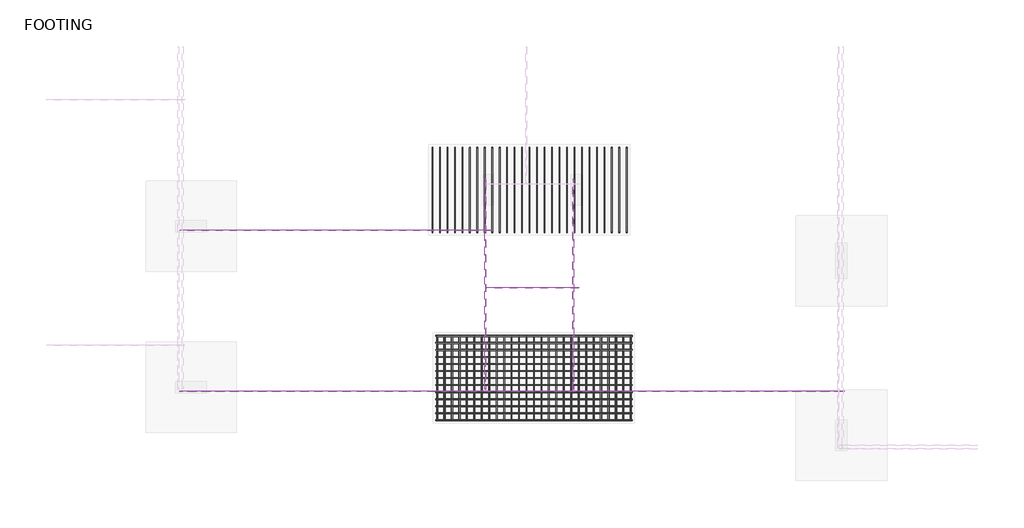
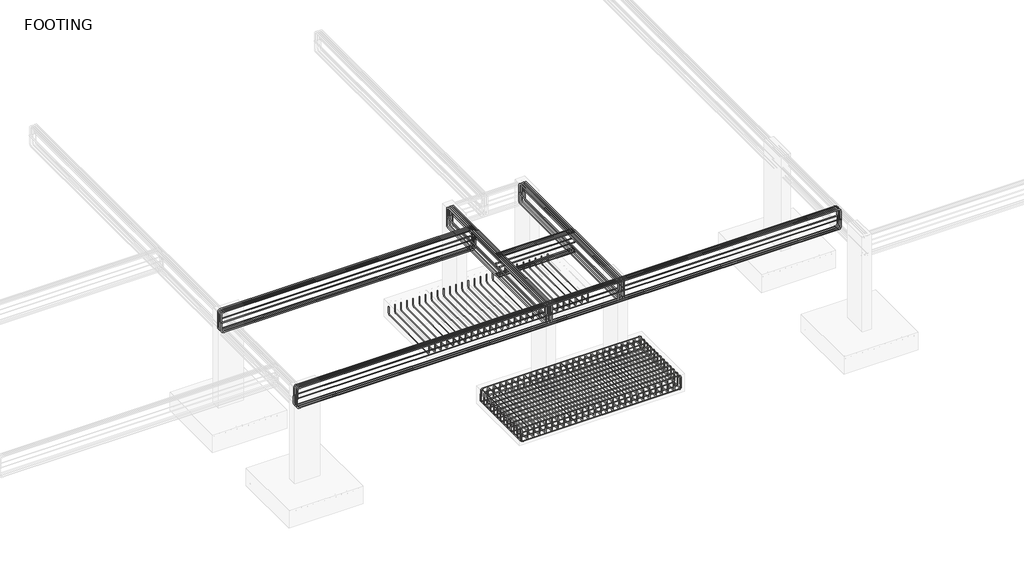
# One storey, part 3 of 12: 20 reinforcing bars.
"""IFC4 building model written with IfcOpenShell, lengths in millimetres."""

from ifc_helpers import new_model, si_unit, point, frame, origin, place, context, project, spatial, polyline, circle_curve, trimmed, segment, composite_curve, source, transform, mapped, element, save
from ifc_brep_helpers import swept_disk

model = new_model("IFC4")

# Units and contexts
model_context = context("Model", 3, world=origin())
ifc_project = project(units=[si_unit("LENGTHUNIT", "METRE", prefix="MILLI")], contexts=[model_context])

# Site, building, storey
site = spatial("IfcSite", under=ifc_project)
building = spatial("IfcBuilding", under=site)
storey = spatial("IfcBuildingStorey", under=building, Name="FOOTING", Elevation=-5638.8)

# Reinforcing bars
placement = place(None, origin())
reinforcing_bar_shape = source(origin(), model_context, "Body", "SolidModel", [
    swept_disk(composite_curve([segment(polyline([(-3549.5501665, -12181.7541655, -5831.4), (-3549.5501665, -12181.7541655, -5978.7)]), True, "CONTINUOUS"), segment(trimmed(circle_curve(frame((-3549.5501665, -12228.1041655, -5978.7), z_axis=(-1.0, 0.0, 0.0), x_axis=(0.0, 46.350000000000364, 0.0)), 46.35), [point((-3549.5501665, -12181.7541655, -5978.7))], [point((-3549.5501665, -12228.1041655, -6025.05))], True, "CARTESIAN"), True, "CONTINUOUS"), segment(polyline([(-3549.5501665, -12228.1041655, -6025.05), (-3549.5501665, -13822.7041655, -6025.05)]), True, "CONTINUOUS"), segment(trimmed(circle_curve(frame((-3549.5501665, -13822.7041655, -5978.7), z_axis=(-1.0, 0.0, 0.0), x_axis=(0.0, 0.0, -46.350000000000364)), 46.35), [point((-3549.5501665, -13822.7041655, -6025.05))], [point((-3549.5501665, -13869.0541655, -5978.7))], True, "CARTESIAN"), True, "CONTINUOUS"), segment(polyline([(-3549.5501665, -13869.0541655, -5978.7), (-3549.5501665, -13869.0541655, -5831.4)]), True, "CONTINUOUS")], self_intersect=False), 6.35),
])
element("IfcReinforcingBar", 1, at=placement, inside=storey, context=model_context, shape_type="MappedRepresentation", body=[
    mapped(reinforcing_bar_shape, transform((0.0, 0.0, 0.0), x_axis=(1.0, 0.0, 0.0), y_axis=(0.0, 1.0, 0.0), z_axis=(0.0, 0.0, 1.0))),
    mapped(reinforcing_bar_shape, transform((148.4113099, 0.0, 0.0), x_axis=(1.0, 0.0, 0.0), y_axis=(0.0, 1.0, 0.0), z_axis=(0.0, 0.0, 1.0))),
    mapped(reinforcing_bar_shape, transform((296.8226198, 0.0, 0.0), x_axis=(1.0, 0.0, 0.0), y_axis=(0.0, 1.0, 0.0), z_axis=(0.0, 0.0, 1.0))),
    mapped(reinforcing_bar_shape, transform((445.2339297, 0.0, 0.0), x_axis=(1.0, 0.0, 0.0), y_axis=(0.0, 1.0, 0.0), z_axis=(0.0, 0.0, 1.0))),
    mapped(reinforcing_bar_shape, transform((593.6452396, 0.0, 0.0), x_axis=(1.0, 0.0, 0.0), y_axis=(0.0, 1.0, 0.0), z_axis=(0.0, 0.0, 1.0))),
    mapped(reinforcing_bar_shape, transform((742.0565495, 0.0, 0.0), x_axis=(1.0, 0.0, 0.0), y_axis=(0.0, 1.0, 0.0), z_axis=(0.0, 0.0, 1.0))),
    mapped(reinforcing_bar_shape, transform((890.4678594, 0.0, 0.0), x_axis=(1.0, 0.0, 0.0), y_axis=(0.0, 1.0, 0.0), z_axis=(0.0, 0.0, 1.0))),
    mapped(reinforcing_bar_shape, transform((1038.8791693, 0.0, 0.0), x_axis=(1.0, 0.0, 0.0), y_axis=(0.0, 1.0, 0.0), z_axis=(0.0, 0.0, 1.0))),
    mapped(reinforcing_bar_shape, transform((1187.2904792, 0.0, 0.0), x_axis=(1.0, 0.0, 0.0), y_axis=(0.0, 1.0, 0.0), z_axis=(0.0, 0.0, 1.0))),
    mapped(reinforcing_bar_shape, transform((1335.7017891, 0.0, 0.0), x_axis=(1.0, 0.0, 0.0), y_axis=(0.0, 1.0, 0.0), z_axis=(0.0, 0.0, 1.0))),
    mapped(reinforcing_bar_shape, transform((1484.113099, 0.0, 0.0), x_axis=(1.0, 0.0, 0.0), y_axis=(0.0, 1.0, 0.0), z_axis=(0.0, 0.0, 1.0))),
    mapped(reinforcing_bar_shape, transform((1632.5244089, 0.0, 0.0), x_axis=(1.0, 0.0, 0.0), y_axis=(0.0, 1.0, 0.0), z_axis=(0.0, 0.0, 1.0))),
    mapped(reinforcing_bar_shape, transform((1780.9357188, 0.0, 0.0), x_axis=(1.0, 0.0, 0.0), y_axis=(0.0, 1.0, 0.0), z_axis=(0.0, 0.0, 1.0))),
    mapped(reinforcing_bar_shape, transform((1929.3470287, 0.0, 0.0), x_axis=(1.0, 0.0, 0.0), y_axis=(0.0, 1.0, 0.0), z_axis=(0.0, 0.0, 1.0))),
    mapped(reinforcing_bar_shape, transform((2077.7583386, 0.0, 0.0), x_axis=(1.0, 0.0, 0.0), y_axis=(0.0, 1.0, 0.0), z_axis=(0.0, 0.0, 1.0))),
    mapped(reinforcing_bar_shape, transform((2226.1696485, 0.0, 0.0), x_axis=(1.0, 0.0, 0.0), y_axis=(0.0, 1.0, 0.0), z_axis=(0.0, 0.0, 1.0))),
    mapped(reinforcing_bar_shape, transform((2374.5809584, 0.0, 0.0), x_axis=(1.0, 0.0, 0.0), y_axis=(0.0, 1.0, 0.0), z_axis=(0.0, 0.0, 1.0))),
    mapped(reinforcing_bar_shape, transform((2522.9922683, 0.0, 0.0), x_axis=(1.0, 0.0, 0.0), y_axis=(0.0, 1.0, 0.0), z_axis=(0.0, 0.0, 1.0))),
    mapped(reinforcing_bar_shape, transform((2671.4035782, 0.0, 0.0), x_axis=(1.0, 0.0, 0.0), y_axis=(0.0, 1.0, 0.0), z_axis=(0.0, 0.0, 1.0))),
    mapped(reinforcing_bar_shape, transform((2819.814888, 0.0, 0.0), x_axis=(1.0, 0.0, 0.0), y_axis=(0.0, 1.0, 0.0), z_axis=(0.0, 0.0, 1.0))),
    mapped(reinforcing_bar_shape, transform((2968.2261979, 0.0, 0.0), x_axis=(1.0, 0.0, 0.0), y_axis=(0.0, 1.0, 0.0), z_axis=(0.0, 0.0, 1.0))),
    mapped(reinforcing_bar_shape, transform((3116.6375078, 0.0, 0.0), x_axis=(1.0, 0.0, 0.0), y_axis=(0.0, 1.0, 0.0), z_axis=(0.0, 0.0, 1.0))),
    mapped(reinforcing_bar_shape, transform((3265.0488177, 0.0, 0.0), x_axis=(1.0, 0.0, 0.0), y_axis=(0.0, 1.0, 0.0), z_axis=(0.0, 0.0, 1.0))),
    mapped(reinforcing_bar_shape, transform((3413.4601276, 0.0, 0.0), x_axis=(1.0, 0.0, 0.0), y_axis=(0.0, 1.0, 0.0), z_axis=(0.0, 0.0, 1.0))),
    mapped(reinforcing_bar_shape, transform((3561.8714375, 0.0, 0.0), x_axis=(1.0, 0.0, 0.0), y_axis=(0.0, 1.0, 0.0), z_axis=(0.0, 0.0, 1.0))),
    mapped(reinforcing_bar_shape, transform((3710.2827474, 0.0, 0.0), x_axis=(1.0, 0.0, 0.0), y_axis=(0.0, 1.0, 0.0), z_axis=(0.0, 0.0, 1.0))),
    mapped(reinforcing_bar_shape, transform((3858.6940573, 0.0, 0.0), x_axis=(1.0, 0.0, 0.0), y_axis=(0.0, 1.0, 0.0), z_axis=(0.0, 0.0, 1.0))),
])
reinforcing_bar_2_shape = source(origin(), model_context, "Body", "SolidModel", [
    swept_disk(composite_curve([segment(polyline([(296.2067827, -12181.7541655, -5901.65), (296.2067827, -12181.7541655, -5754.35)]), True, "CONTINUOUS"), segment(trimmed(circle_curve(frame((296.2067827, -12228.1041655, -5754.35), z_axis=(1.0, 0.0, 0.0), x_axis=(0.0, 46.350000000000364, 0.0)), 46.35), [point((296.2067827, -12181.7541655, -5754.35))], [point((296.2067827, -12228.1041655, -5708.0))], True, "CARTESIAN"), True, "CONTINUOUS"), segment(polyline([(296.2067827, -12228.1041655, -5708.0), (296.2067827, -13822.7041655, -5708.0)]), True, "CONTINUOUS"), segment(trimmed(circle_curve(frame((296.2067827, -13822.7041655, -5754.35), z_axis=(1.0, 0.0, 0.0), x_axis=(0.0, 0.0, 46.350000000000364)), 46.35), [point((296.2067827, -13822.7041655, -5708.0))], [point((296.2067827, -13869.0541655, -5754.35))], True, "CARTESIAN"), True, "CONTINUOUS"), segment(polyline([(296.2067827, -13869.0541655, -5754.35), (296.2067827, -13869.0541655, -5901.65)]), True, "CONTINUOUS")], self_intersect=False), 6.35),
])
element("IfcReinforcingBar", 2, at=placement, inside=storey, context=model_context, shape_type="MappedRepresentation", body=[
    mapped(reinforcing_bar_2_shape, transform((0.0, 0.0, 0.0), x_axis=(1.0, 0.0, 0.0), y_axis=(0.0, 1.0, 0.0), z_axis=(0.0, 0.0, 1.0))),
    mapped(reinforcing_bar_2_shape, transform((-147.4810365, 0.0, 0.0), x_axis=(1.0, 0.0, 0.0), y_axis=(0.0, 1.0, 0.0), z_axis=(0.0, 0.0, 1.0))),
    mapped(reinforcing_bar_2_shape, transform((-294.962073, 0.0, 0.0), x_axis=(1.0, 0.0, 0.0), y_axis=(0.0, 1.0, 0.0), z_axis=(0.0, 0.0, 1.0))),
    mapped(reinforcing_bar_2_shape, transform((-442.4431095, 0.0, 0.0), x_axis=(1.0, 0.0, 0.0), y_axis=(0.0, 1.0, 0.0), z_axis=(0.0, 0.0, 1.0))),
    mapped(reinforcing_bar_2_shape, transform((-589.924146, 0.0, 0.0), x_axis=(1.0, 0.0, 0.0), y_axis=(0.0, 1.0, 0.0), z_axis=(0.0, 0.0, 1.0))),
    mapped(reinforcing_bar_2_shape, transform((-737.4051825, 0.0, 0.0), x_axis=(1.0, 0.0, 0.0), y_axis=(0.0, 1.0, 0.0), z_axis=(0.0, 0.0, 1.0))),
    mapped(reinforcing_bar_2_shape, transform((-884.886219, 0.0, 0.0), x_axis=(1.0, 0.0, 0.0), y_axis=(0.0, 1.0, 0.0), z_axis=(0.0, 0.0, 1.0))),
    mapped(reinforcing_bar_2_shape, transform((-1032.3672556, 0.0, 0.0), x_axis=(1.0, 0.0, 0.0), y_axis=(0.0, 1.0, 0.0), z_axis=(0.0, 0.0, 1.0))),
    mapped(reinforcing_bar_2_shape, transform((-1179.8482921, 0.0, 0.0), x_axis=(1.0, 0.0, 0.0), y_axis=(0.0, 1.0, 0.0), z_axis=(0.0, 0.0, 1.0))),
    mapped(reinforcing_bar_2_shape, transform((-1327.3293286, 0.0, 0.0), x_axis=(1.0, 0.0, 0.0), y_axis=(0.0, 1.0, 0.0), z_axis=(0.0, 0.0, 1.0))),
    mapped(reinforcing_bar_2_shape, transform((-1474.8103651, 0.0, 0.0), x_axis=(1.0, 0.0, 0.0), y_axis=(0.0, 1.0, 0.0), z_axis=(0.0, 0.0, 1.0))),
    mapped(reinforcing_bar_2_shape, transform((-1622.2914016, 0.0, 0.0), x_axis=(1.0, 0.0, 0.0), y_axis=(0.0, 1.0, 0.0), z_axis=(0.0, 0.0, 1.0))),
    mapped(reinforcing_bar_2_shape, transform((-1769.7724381, 0.0, 0.0), x_axis=(1.0, 0.0, 0.0), y_axis=(0.0, 1.0, 0.0), z_axis=(0.0, 0.0, 1.0))),
    mapped(reinforcing_bar_2_shape, transform((-1917.2534746, 0.0, 0.0), x_axis=(1.0, 0.0, 0.0), y_axis=(0.0, 1.0, 0.0), z_axis=(0.0, 0.0, 1.0))),
    mapped(reinforcing_bar_2_shape, transform((-2064.7345111, 0.0, 0.0), x_axis=(1.0, 0.0, 0.0), y_axis=(0.0, 1.0, 0.0), z_axis=(0.0, 0.0, 1.0))),
    mapped(reinforcing_bar_2_shape, transform((-2212.2155476, 0.0, 0.0), x_axis=(1.0, 0.0, 0.0), y_axis=(0.0, 1.0, 0.0), z_axis=(0.0, 0.0, 1.0))),
    mapped(reinforcing_bar_2_shape, transform((-2359.6965841, 0.0, 0.0), x_axis=(1.0, 0.0, 0.0), y_axis=(0.0, 1.0, 0.0), z_axis=(0.0, 0.0, 1.0))),
    mapped(reinforcing_bar_2_shape, transform((-2507.1776206, 0.0, 0.0), x_axis=(1.0, 0.0, 0.0), y_axis=(0.0, 1.0, 0.0), z_axis=(0.0, 0.0, 1.0))),
    mapped(reinforcing_bar_2_shape, transform((-2654.6586571, 0.0, 0.0), x_axis=(1.0, 0.0, 0.0), y_axis=(0.0, 1.0, 0.0), z_axis=(0.0, 0.0, 1.0))),
    mapped(reinforcing_bar_2_shape, transform((-2802.1396936, 0.0, 0.0), x_axis=(1.0, 0.0, 0.0), y_axis=(0.0, 1.0, 0.0), z_axis=(0.0, 0.0, 1.0))),
    mapped(reinforcing_bar_2_shape, transform((-2949.6207301, 0.0, 0.0), x_axis=(1.0, 0.0, 0.0), y_axis=(0.0, 1.0, 0.0), z_axis=(0.0, 0.0, 1.0))),
    mapped(reinforcing_bar_2_shape, transform((-3097.1017667, 0.0, 0.0), x_axis=(1.0, 0.0, 0.0), y_axis=(0.0, 1.0, 0.0), z_axis=(0.0, 0.0, 1.0))),
    mapped(reinforcing_bar_2_shape, transform((-3244.5828032, 0.0, 0.0), x_axis=(1.0, 0.0, 0.0), y_axis=(0.0, 1.0, 0.0), z_axis=(0.0, 0.0, 1.0))),
    mapped(reinforcing_bar_2_shape, transform((-3392.0638397, 0.0, 0.0), x_axis=(1.0, 0.0, 0.0), y_axis=(0.0, 1.0, 0.0), z_axis=(0.0, 0.0, 1.0))),
    mapped(reinforcing_bar_2_shape, transform((-3539.5448762, 0.0, 0.0), x_axis=(1.0, 0.0, 0.0), y_axis=(0.0, 1.0, 0.0), z_axis=(0.0, 0.0, 1.0))),
    mapped(reinforcing_bar_2_shape, transform((-3687.0259127, 0.0, 0.0), x_axis=(1.0, 0.0, 0.0), y_axis=(0.0, 1.0, 0.0), z_axis=(0.0, 0.0, 1.0))),
    mapped(reinforcing_bar_2_shape, transform((-3834.5069492, 0.0, 0.0), x_axis=(1.0, 0.0, 0.0), y_axis=(0.0, 1.0, 0.0), z_axis=(0.0, 0.0, 1.0))),
])
reinforcing_bar_3_shape = source(origin(), model_context, "Body", "SolidModel", [
    swept_disk(composite_curve([segment(polyline([(-3563.3001665, -13869.0541655, -5838.8), (-3563.3001665, -13869.0541655, -5986.1)]), True, "CONTINUOUS"), segment(trimmed(circle_curve(frame((-3516.9501665, -13869.0541655, -5986.1), z_axis=(0.0, -1.0, 0.0), x_axis=(-46.350000000000364, 0.0, 0.0)), 46.35), [point((-3563.3001665, -13869.0541655, -5986.1))], [point((-3516.9501665, -13869.0541655, -6032.45))], True, "CARTESIAN"), True, "CONTINUOUS"), segment(polyline([(-3516.9501665, -13869.0541655, -6032.45), (277.6498335, -13869.0541655, -6032.45)]), True, "CONTINUOUS"), segment(trimmed(circle_curve(frame((277.6498335, -13869.0541655, -5986.1), z_axis=(0.0, -1.0, 0.0), x_axis=(0.0, 0.0, -46.349999999999454)), 46.35), [point((277.6498335, -13869.0541655, -6032.45))], [point((323.9998335, -13869.0541655, -5986.1))], True, "CARTESIAN"), True, "CONTINUOUS"), segment(polyline([(323.9998335, -13869.0541655, -5986.1), (323.9998335, -13869.0541655, -5838.8)]), True, "CONTINUOUS")], self_intersect=False), 6.35),
])
element("IfcReinforcingBar", 3, at=placement, inside=storey, context=model_context, shape_type="MappedRepresentation", body=[
    mapped(reinforcing_bar_3_shape, transform((0.0, 0.0, 0.0), x_axis=(1.0, 0.0, 0.0), y_axis=(0.0, 1.0, 0.0), z_axis=(0.0, 0.0, 1.0))),
    mapped(reinforcing_bar_3_shape, transform((0.0, 140.6083333, 0.0), x_axis=(1.0, 0.0, 0.0), y_axis=(0.0, 1.0, 0.0), z_axis=(0.0, 0.0, 1.0))),
    mapped(reinforcing_bar_3_shape, transform((0.0, 281.2166667, 0.0), x_axis=(1.0, 0.0, 0.0), y_axis=(0.0, 1.0, 0.0), z_axis=(0.0, 0.0, 1.0))),
    mapped(reinforcing_bar_3_shape, transform((0.0, 421.825, 0.0), x_axis=(1.0, 0.0, 0.0), y_axis=(0.0, 1.0, 0.0), z_axis=(0.0, 0.0, 1.0))),
    mapped(reinforcing_bar_3_shape, transform((0.0, 562.4333333, 0.0), x_axis=(1.0, 0.0, 0.0), y_axis=(0.0, 1.0, 0.0), z_axis=(0.0, 0.0, 1.0))),
    mapped(reinforcing_bar_3_shape, transform((0.0, 703.0416667, 0.0), x_axis=(1.0, 0.0, 0.0), y_axis=(0.0, 1.0, 0.0), z_axis=(0.0, 0.0, 1.0))),
    mapped(reinforcing_bar_3_shape, transform((0.0, 843.65, 0.0), x_axis=(1.0, 0.0, 0.0), y_axis=(0.0, 1.0, 0.0), z_axis=(0.0, 0.0, 1.0))),
    mapped(reinforcing_bar_3_shape, transform((0.0, 984.2583333, 0.0), x_axis=(1.0, 0.0, 0.0), y_axis=(0.0, 1.0, 0.0), z_axis=(0.0, 0.0, 1.0))),
    mapped(reinforcing_bar_3_shape, transform((0.0, 1124.8666667, 0.0), x_axis=(1.0, 0.0, 0.0), y_axis=(0.0, 1.0, 0.0), z_axis=(0.0, 0.0, 1.0))),
    mapped(reinforcing_bar_3_shape, transform((0.0, 1265.475, 0.0), x_axis=(1.0, 0.0, 0.0), y_axis=(0.0, 1.0, 0.0), z_axis=(0.0, 0.0, 1.0))),
    mapped(reinforcing_bar_3_shape, transform((0.0, 1406.0833333, 0.0), x_axis=(1.0, 0.0, 0.0), y_axis=(0.0, 1.0, 0.0), z_axis=(0.0, 0.0, 1.0))),
    mapped(reinforcing_bar_3_shape, transform((0.0, 1546.6916667, 0.0), x_axis=(1.0, 0.0, 0.0), y_axis=(0.0, 1.0, 0.0), z_axis=(0.0, 0.0, 1.0))),
    mapped(reinforcing_bar_3_shape, transform((0.0, 1687.3, 0.0), x_axis=(1.0, 0.0, 0.0), y_axis=(0.0, 1.0, 0.0), z_axis=(0.0, 0.0, 1.0))),
])
reinforcing_bar_4_shape = source(origin(), model_context, "Body", "SolidModel", [
    swept_disk(composite_curve([segment(polyline([(323.9998335, -13856.3720387, -5888.8), (323.9998335, -13856.3720387, -5741.5)]), True, "CONTINUOUS"), segment(trimmed(circle_curve(frame((277.6498335, -13856.3720387, -5741.5), z_axis=(0.0, -1.0, 0.0), x_axis=(46.35000000000002, 0.0, 0.0)), 46.35), [point((323.9998335, -13856.3720387, -5741.5))], [point((277.6498335, -13856.3720387, -5695.15))], True, "CARTESIAN"), True, "CONTINUOUS"), segment(polyline([(277.6498335, -13856.3720387, -5695.15), (-3516.9501665, -13856.3720387, -5695.15)]), True, "CONTINUOUS"), segment(trimmed(circle_curve(frame((-3516.9501665, -13856.3720387, -5741.5), z_axis=(0.0, -1.0, 0.0), x_axis=(0.0, 0.0, 46.350000000000364)), 46.35), [point((-3516.9501665, -13856.3720387, -5695.15))], [point((-3563.3001665, -13856.3720387, -5741.5))], True, "CARTESIAN"), True, "CONTINUOUS"), segment(polyline([(-3563.3001665, -13856.3720387, -5741.5), (-3563.3001665, -13856.3720387, -5888.8)]), True, "CONTINUOUS")], self_intersect=False), 6.35),
])
element("IfcReinforcingBar", 4, at=placement, inside=storey, context=model_context, shape_type="MappedRepresentation", body=[
    mapped(reinforcing_bar_4_shape, transform((0.0, 0.0, 0.0), x_axis=(1.0, 0.0, 0.0), y_axis=(0.0, 1.0, 0.0), z_axis=(0.0, 0.0, 1.0))),
    mapped(reinforcing_bar_4_shape, transform((0.0, 138.5098228, 0.0), x_axis=(1.0, 0.0, 0.0), y_axis=(0.0, 1.0, 0.0), z_axis=(0.0, 0.0, 1.0))),
    mapped(reinforcing_bar_4_shape, transform((0.0, 277.0196455, 0.0), x_axis=(1.0, 0.0, 0.0), y_axis=(0.0, 1.0, 0.0), z_axis=(0.0, 0.0, 1.0))),
    mapped(reinforcing_bar_4_shape, transform((0.0, 415.5294683, 0.0), x_axis=(1.0, 0.0, 0.0), y_axis=(0.0, 1.0, 0.0), z_axis=(0.0, 0.0, 1.0))),
    mapped(reinforcing_bar_4_shape, transform((0.0, 554.0392911, 0.0), x_axis=(1.0, 0.0, 0.0), y_axis=(0.0, 1.0, 0.0), z_axis=(0.0, 0.0, 1.0))),
    mapped(reinforcing_bar_4_shape, transform((0.0, 692.5491138, 0.0), x_axis=(1.0, 0.0, 0.0), y_axis=(0.0, 1.0, 0.0), z_axis=(0.0, 0.0, 1.0))),
    mapped(reinforcing_bar_4_shape, transform((0.0, 831.0589366, 0.0), x_axis=(1.0, 0.0, 0.0), y_axis=(0.0, 1.0, 0.0), z_axis=(0.0, 0.0, 1.0))),
    mapped(reinforcing_bar_4_shape, transform((0.0, 969.5687594, 0.0), x_axis=(1.0, 0.0, 0.0), y_axis=(0.0, 1.0, 0.0), z_axis=(0.0, 0.0, 1.0))),
    mapped(reinforcing_bar_4_shape, transform((0.0, 1108.0785821, 0.0), x_axis=(1.0, 0.0, 0.0), y_axis=(0.0, 1.0, 0.0), z_axis=(0.0, 0.0, 1.0))),
    mapped(reinforcing_bar_4_shape, transform((0.0, 1246.5884049, 0.0), x_axis=(1.0, 0.0, 0.0), y_axis=(0.0, 1.0, 0.0), z_axis=(0.0, 0.0, 1.0))),
    mapped(reinforcing_bar_4_shape, transform((0.0, 1385.0982277, 0.0), x_axis=(1.0, 0.0, 0.0), y_axis=(0.0, 1.0, 0.0), z_axis=(0.0, 0.0, 1.0))),
    mapped(reinforcing_bar_4_shape, transform((0.0, 1523.6080504, 0.0), x_axis=(1.0, 0.0, 0.0), y_axis=(0.0, 1.0, 0.0), z_axis=(0.0, 0.0, 1.0))),
    mapped(reinforcing_bar_4_shape, transform((0.0, 1662.1178732, 0.0), x_axis=(1.0, 0.0, 0.0), y_axis=(0.0, 1.0, 0.0), z_axis=(0.0, 0.0, 1.0))),
])
reinforcing_bar_5_shape = source(origin(), model_context, "Body", "SolidModel", [
    swept_disk(composite_curve([segment(polyline([(-3636.7501665, -8447.9541655, -5831.4), (-3636.7501665, -8447.9541655, -5978.7)]), True, "CONTINUOUS"), segment(trimmed(circle_curve(frame((-3636.7501665, -8494.3041655, -5978.7), z_axis=(-1.0, 0.0, 0.0), x_axis=(0.0, 46.350000000000364, 0.0)), 46.35), [point((-3636.7501665, -8447.9541655, -5978.7))], [point((-3636.7501665, -8494.3041655, -6025.05))], True, "CARTESIAN"), True, "CONTINUOUS"), segment(polyline([(-3636.7501665, -8494.3041655, -6025.05), (-3636.7501665, -10088.9041655, -6025.05)]), True, "CONTINUOUS"), segment(trimmed(circle_curve(frame((-3636.7501665, -10088.9041655, -5978.7), z_axis=(-1.0, 0.0, 0.0), x_axis=(0.0, 0.0, -46.350000000000364)), 46.35), [point((-3636.7501665, -10088.9041655, -6025.05))], [point((-3636.7501665, -10135.2541655, -5978.7))], True, "CARTESIAN"), True, "CONTINUOUS"), segment(polyline([(-3636.7501665, -10135.2541655, -5978.7), (-3636.7501665, -10135.2541655, -5831.4)]), True, "CONTINUOUS")], self_intersect=False), 6.35),
])
element("IfcReinforcingBar", 5, at=placement, inside=storey, context=model_context, shape_type="MappedRepresentation", body=[
    mapped(reinforcing_bar_5_shape, transform((0.0, 0.0, 0.0), x_axis=(1.0, 0.0, 0.0), y_axis=(0.0, 1.0, 0.0), z_axis=(0.0, 0.0, 1.0))),
    mapped(reinforcing_bar_5_shape, transform((148.4113099, 0.0, 0.0), x_axis=(1.0, 0.0, 0.0), y_axis=(0.0, 1.0, 0.0), z_axis=(0.0, 0.0, 1.0))),
    mapped(reinforcing_bar_5_shape, transform((296.8226198, 0.0, 0.0), x_axis=(1.0, 0.0, 0.0), y_axis=(0.0, 1.0, 0.0), z_axis=(0.0, 0.0, 1.0))),
    mapped(reinforcing_bar_5_shape, transform((445.2339297, 0.0, 0.0), x_axis=(1.0, 0.0, 0.0), y_axis=(0.0, 1.0, 0.0), z_axis=(0.0, 0.0, 1.0))),
    mapped(reinforcing_bar_5_shape, transform((593.6452396, 0.0, 0.0), x_axis=(1.0, 0.0, 0.0), y_axis=(0.0, 1.0, 0.0), z_axis=(0.0, 0.0, 1.0))),
    mapped(reinforcing_bar_5_shape, transform((742.0565495, 0.0, 0.0), x_axis=(1.0, 0.0, 0.0), y_axis=(0.0, 1.0, 0.0), z_axis=(0.0, 0.0, 1.0))),
    mapped(reinforcing_bar_5_shape, transform((890.4678594, 0.0, 0.0), x_axis=(1.0, 0.0, 0.0), y_axis=(0.0, 1.0, 0.0), z_axis=(0.0, 0.0, 1.0))),
    mapped(reinforcing_bar_5_shape, transform((1038.8791693, 0.0, 0.0), x_axis=(1.0, 0.0, 0.0), y_axis=(0.0, 1.0, 0.0), z_axis=(0.0, 0.0, 1.0))),
    mapped(reinforcing_bar_5_shape, transform((1187.2904792, 0.0, 0.0), x_axis=(1.0, 0.0, 0.0), y_axis=(0.0, 1.0, 0.0), z_axis=(0.0, 0.0, 1.0))),
    mapped(reinforcing_bar_5_shape, transform((1335.7017891, 0.0, 0.0), x_axis=(1.0, 0.0, 0.0), y_axis=(0.0, 1.0, 0.0), z_axis=(0.0, 0.0, 1.0))),
    mapped(reinforcing_bar_5_shape, transform((1484.113099, 0.0, 0.0), x_axis=(1.0, 0.0, 0.0), y_axis=(0.0, 1.0, 0.0), z_axis=(0.0, 0.0, 1.0))),
    mapped(reinforcing_bar_5_shape, transform((1632.5244089, 0.0, 0.0), x_axis=(1.0, 0.0, 0.0), y_axis=(0.0, 1.0, 0.0), z_axis=(0.0, 0.0, 1.0))),
    mapped(reinforcing_bar_5_shape, transform((1780.9357188, 0.0, 0.0), x_axis=(1.0, 0.0, 0.0), y_axis=(0.0, 1.0, 0.0), z_axis=(0.0, 0.0, 1.0))),
    mapped(reinforcing_bar_5_shape, transform((1929.3470287, 0.0, 0.0), x_axis=(1.0, 0.0, 0.0), y_axis=(0.0, 1.0, 0.0), z_axis=(0.0, 0.0, 1.0))),
    mapped(reinforcing_bar_5_shape, transform((2077.7583386, 0.0, 0.0), x_axis=(1.0, 0.0, 0.0), y_axis=(0.0, 1.0, 0.0), z_axis=(0.0, 0.0, 1.0))),
    mapped(reinforcing_bar_5_shape, transform((2226.1696485, 0.0, 0.0), x_axis=(1.0, 0.0, 0.0), y_axis=(0.0, 1.0, 0.0), z_axis=(0.0, 0.0, 1.0))),
    mapped(reinforcing_bar_5_shape, transform((2374.5809584, 0.0, 0.0), x_axis=(1.0, 0.0, 0.0), y_axis=(0.0, 1.0, 0.0), z_axis=(0.0, 0.0, 1.0))),
    mapped(reinforcing_bar_5_shape, transform((2522.9922683, 0.0, 0.0), x_axis=(1.0, 0.0, 0.0), y_axis=(0.0, 1.0, 0.0), z_axis=(0.0, 0.0, 1.0))),
    mapped(reinforcing_bar_5_shape, transform((2671.4035782, 0.0, 0.0), x_axis=(1.0, 0.0, 0.0), y_axis=(0.0, 1.0, 0.0), z_axis=(0.0, 0.0, 1.0))),
    mapped(reinforcing_bar_5_shape, transform((2819.814888, 0.0, 0.0), x_axis=(1.0, 0.0, 0.0), y_axis=(0.0, 1.0, 0.0), z_axis=(0.0, 0.0, 1.0))),
    mapped(reinforcing_bar_5_shape, transform((2968.2261979, 0.0, 0.0), x_axis=(1.0, 0.0, 0.0), y_axis=(0.0, 1.0, 0.0), z_axis=(0.0, 0.0, 1.0))),
    mapped(reinforcing_bar_5_shape, transform((3116.6375078, 0.0, 0.0), x_axis=(1.0, 0.0, 0.0), y_axis=(0.0, 1.0, 0.0), z_axis=(0.0, 0.0, 1.0))),
    mapped(reinforcing_bar_5_shape, transform((3265.0488177, 0.0, 0.0), x_axis=(1.0, 0.0, 0.0), y_axis=(0.0, 1.0, 0.0), z_axis=(0.0, 0.0, 1.0))),
    mapped(reinforcing_bar_5_shape, transform((3413.4601276, 0.0, 0.0), x_axis=(1.0, 0.0, 0.0), y_axis=(0.0, 1.0, 0.0), z_axis=(0.0, 0.0, 1.0))),
    mapped(reinforcing_bar_5_shape, transform((3561.8714375, 0.0, 0.0), x_axis=(1.0, 0.0, 0.0), y_axis=(0.0, 1.0, 0.0), z_axis=(0.0, 0.0, 1.0))),
    mapped(reinforcing_bar_5_shape, transform((3710.2827474, 0.0, 0.0), x_axis=(1.0, 0.0, 0.0), y_axis=(0.0, 1.0, 0.0), z_axis=(0.0, 0.0, 1.0))),
    mapped(reinforcing_bar_5_shape, transform((3858.6940573, 0.0, 0.0), x_axis=(1.0, 0.0, 0.0), y_axis=(0.0, 1.0, 0.0), z_axis=(0.0, 0.0, 1.0))),
])
reinforcing_bar_6_shape = source(origin(), model_context, "Body", "SolidModel", [
    swept_disk(composite_curve([segment(polyline([(-2447.8001665, -13248.4002615, -3500.1457532), (-2447.8001665, -9081.1442712, -3500.1457532)]), True, "CONTINUOUS")], self_intersect=False), 7.95),
])
element("IfcReinforcingBar", 6, at=placement, inside=storey, context=model_context, shape_type="MappedRepresentation", body=[
    mapped(reinforcing_bar_6_shape, transform((0.0, 0.0, 0.0), x_axis=(1.0, 0.0, 0.0), y_axis=(0.0, 1.0, 0.0), z_axis=(0.0, 0.0, 1.0))),
    mapped(reinforcing_bar_6_shape, transform((-143.7, 0.0, 0.0), x_axis=(1.0, 0.0, 0.0), y_axis=(0.0, 1.0, 0.0), z_axis=(0.0, 0.0, 1.0))),
])
reinforcing_bar_7_shape = source(origin(), model_context, "Body", "SolidModel", [
    swept_disk(composite_curve([segment(polyline([(-2451.3295298, -13245.6338123, -3488.4293633), (-2451.3295298, -13245.6338123, -3301.8293633)]), True, "CONTINUOUS"), segment(trimmed(circle_curve(frame((-2451.3295298, -13190.1838123, -3301.8293633), z_axis=(-1.0, 0.0, 0.0), x_axis=(0.0, -55.45000000000073, 0.0)), 55.45), [point((-2451.3295298, -13245.6338123, -3301.8293633))], [point((-2451.3295298, -13190.1838123, -3246.3793633))], True, "CARTESIAN"), True, "CONTINUOUS"), segment(polyline([(-2451.3295298, -13190.1838123, -3246.3793633), (-2451.3295298, -9138.5286827, -3246.3793633)]), True, "CONTINUOUS"), segment(trimmed(circle_curve(frame((-2451.3295298, -9138.5286827, -3301.8293633), z_axis=(-1.0, 0.0, 0.0), x_axis=(0.0, 0.0, 55.44999999999982)), 55.45), [point((-2451.3295298, -9138.5286827, -3246.3793633))], [point((-2451.3295298, -9083.0786827, -3301.8293633))], True, "CARTESIAN"), True, "CONTINUOUS"), segment(polyline([(-2451.3295298, -9083.0786827, -3301.8293633), (-2451.3295298, -9083.0786827, -3488.4293633)]), True, "CONTINUOUS")], self_intersect=False), 7.95),
])
element("IfcReinforcingBar", 7, at=placement, inside=storey, context=model_context, shape_type="MappedRepresentation", body=[
    mapped(reinforcing_bar_7_shape, transform((0.0, 0.0, 0.0), x_axis=(1.0, 0.0, 0.0), y_axis=(0.0, 1.0, 0.0), z_axis=(0.0, 0.0, 1.0))),
    mapped(reinforcing_bar_7_shape, transform((-45.5470911, 0.0, 0.0), x_axis=(1.0, 0.0, 0.0), y_axis=(0.0, 1.0, 0.0), z_axis=(0.0, 0.0, 1.0))),
    mapped(reinforcing_bar_7_shape, transform((-91.0941823, 0.0, 0.0), x_axis=(1.0, 0.0, 0.0), y_axis=(0.0, 1.0, 0.0), z_axis=(0.0, 0.0, 1.0))),
    mapped(reinforcing_bar_7_shape, transform((-136.6412734, 0.0, 0.0), x_axis=(1.0, 0.0, 0.0), y_axis=(0.0, 1.0, 0.0), z_axis=(0.0, 0.0, 1.0))),
])
reinforcing_bar_8_shape = source(origin(), model_context, "Body", "SolidModel", [
    swept_disk(composite_curve([segment(polyline([(-2451.3295298, -13243.1472317, -3512.3706367), (-2451.3295298, -13243.1472317, -3698.9706367)]), True, "CONTINUOUS"), segment(trimmed(circle_curve(frame((-2451.3295298, -13187.6972317, -3698.9706367), z_axis=(1.0, 0.0, 0.0), x_axis=(0.0, -55.45000000000073, 0.0)), 55.45), [point((-2451.3295298, -13243.1472317, -3698.9706367))], [point((-2451.3295298, -13187.6972317, -3754.4206367))], True, "CARTESIAN"), True, "CONTINUOUS"), segment(polyline([(-2451.3295298, -13187.6972317, -3754.4206367), (-2451.3295298, -9131.6689879, -3754.4206367)]), True, "CONTINUOUS"), segment(trimmed(circle_curve(frame((-2451.3295298, -9131.6689879, -3698.9706367), z_axis=(1.0, 0.0, 0.0), x_axis=(0.0, 0.0, -55.45000000000027)), 55.45), [point((-2451.3295298, -9131.6689879, -3754.4206367))], [point((-2451.3295298, -9076.2189879, -3698.9706367))], True, "CARTESIAN"), True, "CONTINUOUS"), segment(polyline([(-2451.3295298, -9076.2189879, -3698.9706367), (-2451.3295298, -9076.2189879, -3512.3706367)]), True, "CONTINUOUS")], self_intersect=False), 7.95),
])
element("IfcReinforcingBar", 8, at=placement, inside=storey, context=model_context, shape_type="MappedRepresentation", body=[
    mapped(reinforcing_bar_8_shape, transform((0.0, 0.0, 0.0), x_axis=(1.0, 0.0, 0.0), y_axis=(0.0, 1.0, 0.0), z_axis=(0.0, 0.0, 1.0))),
    mapped(reinforcing_bar_8_shape, transform((-68.3206367, 0.0, 0.0), x_axis=(1.0, 0.0, 0.0), y_axis=(0.0, 1.0, 0.0), z_axis=(0.0, 0.0, 1.0))),
    mapped(reinforcing_bar_8_shape, transform((-136.6412734, 0.0, 0.0), x_axis=(1.0, 0.0, 0.0), y_axis=(0.0, 1.0, 0.0), z_axis=(0.0, 0.0, 1.0))),
])
reinforcing_bar_9_shape = source(origin(), model_context, "Body", "SolidModel", [
    swept_disk(composite_curve([segment(polyline([(-695.2001665, -13248.4002615, -3500.1457532), (-695.2001665, -9081.1442712, -3500.1457532)]), True, "CONTINUOUS")], self_intersect=False), 7.95),
])
element("IfcReinforcingBar", 9, at=placement, inside=storey, context=model_context, shape_type="MappedRepresentation", body=[
    mapped(reinforcing_bar_9_shape, transform((0.0, 0.0, 0.0), x_axis=(1.0, 0.0, 0.0), y_axis=(0.0, 1.0, 0.0), z_axis=(0.0, 0.0, 1.0))),
    mapped(reinforcing_bar_9_shape, transform((-143.7, 0.0, 0.0), x_axis=(1.0, 0.0, 0.0), y_axis=(0.0, 1.0, 0.0), z_axis=(0.0, 0.0, 1.0))),
])
reinforcing_bar_10_shape = source(origin(), model_context, "Body", "SolidModel", [
    swept_disk(composite_curve([segment(polyline([(-698.7295298, -13245.6338123, -3488.4293633), (-698.7295298, -13245.6338123, -3301.8293633)]), True, "CONTINUOUS"), segment(trimmed(circle_curve(frame((-698.7295298, -13190.1838123, -3301.8293633), z_axis=(-1.0, 0.0, 0.0), x_axis=(0.0, -55.45000000000073, 0.0)), 55.45), [point((-698.7295298, -13245.6338123, -3301.8293633))], [point((-698.7295298, -13190.1838123, -3246.3793633))], True, "CARTESIAN"), True, "CONTINUOUS"), segment(polyline([(-698.7295298, -13190.1838123, -3246.3793633), (-698.7295298, -9138.5286827, -3246.3793633)]), True, "CONTINUOUS"), segment(trimmed(circle_curve(frame((-698.7295298, -9138.5286827, -3301.8293633), z_axis=(-1.0, 0.0, 0.0), x_axis=(0.0, 0.0, 55.44999999999982)), 55.45), [point((-698.7295298, -9138.5286827, -3246.3793633))], [point((-698.7295298, -9083.0786827, -3301.8293633))], True, "CARTESIAN"), True, "CONTINUOUS"), segment(polyline([(-698.7295298, -9083.0786827, -3301.8293633), (-698.7295298, -9083.0786827, -3488.4293633)]), True, "CONTINUOUS")], self_intersect=False), 7.95),
])
element("IfcReinforcingBar", 10, at=placement, inside=storey, context=model_context, shape_type="MappedRepresentation", body=[
    mapped(reinforcing_bar_10_shape, transform((0.0, 0.0, 0.0), x_axis=(1.0, 0.0, 0.0), y_axis=(0.0, 1.0, 0.0), z_axis=(0.0, 0.0, 1.0))),
    mapped(reinforcing_bar_10_shape, transform((-45.5470911, 0.0, 0.0), x_axis=(1.0, 0.0, 0.0), y_axis=(0.0, 1.0, 0.0), z_axis=(0.0, 0.0, 1.0))),
    mapped(reinforcing_bar_10_shape, transform((-91.0941823, 0.0, 0.0), x_axis=(1.0, 0.0, 0.0), y_axis=(0.0, 1.0, 0.0), z_axis=(0.0, 0.0, 1.0))),
    mapped(reinforcing_bar_10_shape, transform((-136.6412734, 0.0, 0.0), x_axis=(1.0, 0.0, 0.0), y_axis=(0.0, 1.0, 0.0), z_axis=(0.0, 0.0, 1.0))),
])
reinforcing_bar_11_shape = source(origin(), model_context, "Body", "SolidModel", [
    swept_disk(composite_curve([segment(polyline([(-698.7295298, -13243.1472317, -3512.3706367), (-698.7295298, -13243.1472317, -3698.9706367)]), True, "CONTINUOUS"), segment(trimmed(circle_curve(frame((-698.7295298, -13187.6972317, -3698.9706367), z_axis=(1.0, 0.0, 0.0), x_axis=(0.0, -55.45000000000073, 0.0)), 55.45), [point((-698.7295298, -13243.1472317, -3698.9706367))], [point((-698.7295298, -13187.6972317, -3754.4206367))], True, "CARTESIAN"), True, "CONTINUOUS"), segment(polyline([(-698.7295298, -13187.6972317, -3754.4206367), (-698.7295298, -9131.6689879, -3754.4206367)]), True, "CONTINUOUS"), segment(trimmed(circle_curve(frame((-698.7295298, -9131.6689879, -3698.9706367), z_axis=(1.0, 0.0, 0.0), x_axis=(0.0, 0.0, -55.45000000000027)), 55.45), [point((-698.7295298, -9131.6689879, -3754.4206367))], [point((-698.7295298, -9076.2189879, -3698.9706367))], True, "CARTESIAN"), True, "CONTINUOUS"), segment(polyline([(-698.7295298, -9076.2189879, -3698.9706367), (-698.7295298, -9076.2189879, -3512.3706367)]), True, "CONTINUOUS")], self_intersect=False), 7.95),
])
element("IfcReinforcingBar", 11, at=placement, inside=storey, context=model_context, shape_type="MappedRepresentation", body=[
    mapped(reinforcing_bar_11_shape, transform((0.0, 0.0, 0.0), x_axis=(1.0, 0.0, 0.0), y_axis=(0.0, 1.0, 0.0), z_axis=(0.0, 0.0, 1.0))),
    mapped(reinforcing_bar_11_shape, transform((-68.3206367, 0.0, 0.0), x_axis=(1.0, 0.0, 0.0), y_axis=(0.0, 1.0, 0.0), z_axis=(0.0, 0.0, 1.0))),
    mapped(reinforcing_bar_11_shape, transform((-136.6412734, 0.0, 0.0), x_axis=(1.0, 0.0, 0.0), y_axis=(0.0, 1.0, 0.0), z_axis=(0.0, 0.0, 1.0))),
])
reinforcing_bar_12_shape = source(origin(), model_context, "Body", "SolidModel", [
    swept_disk(composite_curve([segment(polyline([(4534.0815103, -13284.2248022, -3488.4293633), (4534.0815103, -13284.2248022, -3301.8293633)]), True, "CONTINUOUS"), segment(trimmed(circle_curve(frame((4478.6315103, -13284.2248022, -3301.8293633), z_axis=(0.0, -1.0, 0.0), x_axis=(55.45000000000073, 0.0, 0.0)), 55.45), [point((4534.0815103, -13284.2248022, -3301.8293633))], [point((4478.6315103, -13284.2248022, -3246.3793633))], True, "CARTESIAN"), True, "CONTINUOUS"), segment(polyline([(4478.6315103, -13284.2248022, -3246.3793633), (-8586.7278739, -13284.2248022, -3246.3793633)]), True, "CONTINUOUS"), segment(trimmed(circle_curve(frame((-8586.7278739, -13284.2248022, -3301.8293633), z_axis=(0.0, -1.0, 0.0), x_axis=(0.0, 0.0, 55.44999999999982)), 55.45), [point((-8586.7278739, -13284.2248022, -3246.3793633))], [point((-8642.1778739, -13284.2248022, -3301.8293633))], True, "CARTESIAN"), True, "CONTINUOUS"), segment(polyline([(-8642.1778739, -13284.2248022, -3301.8293633), (-8642.1778739, -13284.2248022, -3488.4293633)]), True, "CONTINUOUS")], self_intersect=False), 7.95),
])
element("IfcReinforcingBar", 12, at=placement, inside=storey, context=model_context, shape_type="MappedRepresentation", body=[
    mapped(reinforcing_bar_12_shape, transform((0.0, 0.0, 0.0), x_axis=(1.0, 0.0, 0.0), y_axis=(0.0, 1.0, 0.0), z_axis=(0.0, 0.0, 1.0))),
    mapped(reinforcing_bar_12_shape, transform((0.0, 45.5470911, 0.0), x_axis=(1.0, 0.0, 0.0), y_axis=(0.0, 1.0, 0.0), z_axis=(0.0, 0.0, 1.0))),
    mapped(reinforcing_bar_12_shape, transform((0.0, 91.0941823, 0.0), x_axis=(1.0, 0.0, 0.0), y_axis=(0.0, 1.0, 0.0), z_axis=(0.0, 0.0, 1.0))),
    mapped(reinforcing_bar_12_shape, transform((0.0, 136.6412734, 0.0), x_axis=(1.0, 0.0, 0.0), y_axis=(0.0, 1.0, 0.0), z_axis=(0.0, 0.0, 1.0))),
])
reinforcing_bar_13_shape = source(origin(), model_context, "Body", "SolidModel", [
    swept_disk(composite_curve([segment(polyline([(4533.1268571, -13144.0541655, -3500.4), (-8648.5784725, -13144.0541655, -3500.4)]), True, "CONTINUOUS")], self_intersect=False), 7.95),
])
element("IfcReinforcingBar", 13, at=placement, inside=storey, context=model_context, shape_type="MappedRepresentation", body=[
    mapped(reinforcing_bar_13_shape, transform((0.0, 0.0, 0.0), x_axis=(1.0, 0.0, 0.0), y_axis=(0.0, 1.0, 0.0), z_axis=(0.0, 0.0, 1.0))),
    mapped(reinforcing_bar_13_shape, transform((0.0, -143.7, 0.0), x_axis=(1.0, 0.0, 0.0), y_axis=(0.0, 1.0, 0.0), z_axis=(0.0, 0.0, 1.0))),
])
reinforcing_bar_14_shape = source(origin(), model_context, "Body", "SolidModel", [
    swept_disk(composite_curve([segment(polyline([(4537.7684992, -13284.2248022, -3512.3706367), (4537.7684992, -13284.2248022, -3698.9706367)]), True, "CONTINUOUS"), segment(trimmed(circle_curve(frame((4482.3184992, -13284.2248022, -3698.9706367), z_axis=(0.0, 1.0, 0.0), x_axis=(55.45000000000073, 0.0, 0.0)), 55.45), [point((4537.7684992, -13284.2248022, -3698.9706367))], [point((4482.3184992, -13284.2248022, -3754.4206367))], True, "CARTESIAN"), True, "CONTINUOUS"), segment(polyline([(4482.3184992, -13284.2248022, -3754.4206367), (-8596.16362, -13284.2248022, -3754.4206367)]), True, "CONTINUOUS"), segment(trimmed(circle_curve(frame((-8596.16362, -13284.2248022, -3698.9706367), z_axis=(0.0, 1.0, 0.0), x_axis=(0.0, 0.0, -55.45000000000027)), 55.45), [point((-8596.16362, -13284.2248022, -3754.4206367))], [point((-8651.61362, -13284.2248022, -3698.9706367))], True, "CARTESIAN"), True, "CONTINUOUS"), segment(polyline([(-8651.61362, -13284.2248022, -3698.9706367), (-8651.61362, -13284.2248022, -3512.3706367)]), True, "CONTINUOUS")], self_intersect=False), 7.95),
])
element("IfcReinforcingBar", 14, at=placement, inside=storey, context=model_context, shape_type="MappedRepresentation", body=[
    mapped(reinforcing_bar_14_shape, transform((0.0, 0.0, 0.0), x_axis=(1.0, 0.0, 0.0), y_axis=(0.0, 1.0, 0.0), z_axis=(0.0, 0.0, 1.0))),
    mapped(reinforcing_bar_14_shape, transform((0.0, 68.3206367, 0.0), x_axis=(1.0, 0.0, 0.0), y_axis=(0.0, 1.0, 0.0), z_axis=(0.0, 0.0, 1.0))),
    mapped(reinforcing_bar_14_shape, transform((0.0, 136.6412734, 0.0), x_axis=(1.0, 0.0, 0.0), y_axis=(0.0, 1.0, 0.0), z_axis=(0.0, 0.0, 1.0))),
])
reinforcing_bar_15_shape = source(origin(), model_context, "Body", "SolidModel", [
    swept_disk(composite_curve([segment(polyline([(-2476.7617951, -10083.8248022, -3488.4293633), (-2476.7617951, -10083.8248022, -3301.8293633)]), True, "CONTINUOUS"), segment(trimmed(circle_curve(frame((-2532.2117951, -10083.8248022, -3301.8293633), z_axis=(0.0, -1.0, 0.0), x_axis=(55.44999999999982, 0.0, 0.0)), 55.45), [point((-2476.7617951, -10083.8248022, -3301.8293633))], [point((-2532.2117951, -10083.8248022, -3246.3793633))], True, "CARTESIAN"), True, "CONTINUOUS"), segment(polyline([(-2532.2117951, -10083.8248022, -3246.3793633), (-8586.7278739, -10083.8248022, -3246.3793633)]), True, "CONTINUOUS"), segment(trimmed(circle_curve(frame((-8586.7278739, -10083.8248022, -3301.8293633), z_axis=(0.0, -1.0, 0.0), x_axis=(0.0, 0.0, 55.44999999999982)), 55.45), [point((-8586.7278739, -10083.8248022, -3246.3793633))], [point((-8642.1778739, -10083.8248022, -3301.8293633))], True, "CARTESIAN"), True, "CONTINUOUS"), segment(polyline([(-8642.1778739, -10083.8248022, -3301.8293633), (-8642.1778739, -10083.8248022, -3488.4293633)]), True, "CONTINUOUS")], self_intersect=False), 7.95),
])
element("IfcReinforcingBar", 15, at=placement, inside=storey, context=model_context, shape_type="MappedRepresentation", body=[
    mapped(reinforcing_bar_15_shape, transform((0.0, 0.0, 0.0), x_axis=(1.0, 0.0, 0.0), y_axis=(0.0, 1.0, 0.0), z_axis=(0.0, 0.0, 1.0))),
    mapped(reinforcing_bar_15_shape, transform((0.0, 45.5470911, 0.0), x_axis=(1.0, 0.0, 0.0), y_axis=(0.0, 1.0, 0.0), z_axis=(0.0, 0.0, 1.0))),
    mapped(reinforcing_bar_15_shape, transform((0.0, 91.0941823, 0.0), x_axis=(1.0, 0.0, 0.0), y_axis=(0.0, 1.0, 0.0), z_axis=(0.0, 0.0, 1.0))),
    mapped(reinforcing_bar_15_shape, transform((0.0, 136.6412734, 0.0), x_axis=(1.0, 0.0, 0.0), y_axis=(0.0, 1.0, 0.0), z_axis=(0.0, 0.0, 1.0))),
])
reinforcing_bar_16_shape = source(origin(), model_context, "Body", "SolidModel", [
    swept_disk(composite_curve([segment(polyline([(-2476.0534915, -9943.6541655, -3500.4), (-8643.7505131, -9943.6541655, -3500.4)]), True, "CONTINUOUS")], self_intersect=False), 7.95),
])
element("IfcReinforcingBar", 16, at=placement, inside=storey, context=model_context, shape_type="MappedRepresentation", body=[
    mapped(reinforcing_bar_16_shape, transform((0.0, 0.0, 0.0), x_axis=(1.0, 0.0, 0.0), y_axis=(0.0, 1.0, 0.0), z_axis=(0.0, 0.0, 1.0))),
    mapped(reinforcing_bar_16_shape, transform((0.0, -143.7, 0.0), x_axis=(1.0, 0.0, 0.0), y_axis=(0.0, 1.0, 0.0), z_axis=(0.0, 0.0, 1.0))),
])
reinforcing_bar_17_shape = source(origin(), model_context, "Body", "SolidModel", [
    swept_disk(composite_curve([segment(polyline([(-2483.6650589, -10083.8248022, -3512.3706367), (-2483.6650589, -10083.8248022, -3698.9706367)]), True, "CONTINUOUS"), segment(trimmed(circle_curve(frame((-2539.1150589, -10083.8248022, -3698.9706367), z_axis=(0.0, 1.0, 0.0), x_axis=(55.44999999999982, 0.0, 0.0)), 55.45), [point((-2483.6650589, -10083.8248022, -3698.9706367))], [point((-2539.1150589, -10083.8248022, -3754.4206367))], True, "CARTESIAN"), True, "CONTINUOUS"), segment(polyline([(-2539.1150589, -10083.8248022, -3754.4206367), (-8586.5864851, -10083.8248022, -3754.4206367)]), True, "CONTINUOUS"), segment(trimmed(circle_curve(frame((-8586.5864851, -10083.8248022, -3698.9706367), z_axis=(0.0, 1.0, 0.0), x_axis=(0.0, 0.0, -55.45000000000027)), 55.45), [point((-8586.5864851, -10083.8248022, -3754.4206367))], [point((-8642.0364851, -10083.8248022, -3698.9706367))], True, "CARTESIAN"), True, "CONTINUOUS"), segment(polyline([(-8642.0364851, -10083.8248022, -3698.9706367), (-8642.0364851, -10083.8248022, -3512.3706367)]), True, "CONTINUOUS")], self_intersect=False), 7.95),
])
element("IfcReinforcingBar", 17, at=placement, inside=storey, context=model_context, shape_type="MappedRepresentation", body=[
    mapped(reinforcing_bar_17_shape, transform((0.0, 0.0, 0.0), x_axis=(1.0, 0.0, 0.0), y_axis=(0.0, 1.0, 0.0), z_axis=(0.0, 0.0, 1.0))),
    mapped(reinforcing_bar_17_shape, transform((0.0, 68.3206367, 0.0), x_axis=(1.0, 0.0, 0.0), y_axis=(0.0, 1.0, 0.0), z_axis=(0.0, 0.0, 1.0))),
    mapped(reinforcing_bar_17_shape, transform((0.0, 136.6412734, 0.0), x_axis=(1.0, 0.0, 0.0), y_axis=(0.0, 1.0, 0.0), z_axis=(0.0, 0.0, 1.0))),
])
reinforcing_bar_18_shape = source(origin(), model_context, "Body", "SolidModel", [
    swept_disk(composite_curve([segment(polyline([(-2554.3135126, -11230.3541655, -3500.4), (-738.7962383, -11230.3541655, -3500.4)]), True, "CONTINUOUS")], self_intersect=False), 7.95),
])
element("IfcReinforcingBar", 18, at=placement, inside=storey, context=model_context, shape_type="MappedRepresentation", body=[
    mapped(reinforcing_bar_18_shape, transform((0.0, 0.0, 0.0), x_axis=(1.0, 0.0, 0.0), y_axis=(0.0, 1.0, 0.0), z_axis=(0.0, 0.0, 1.0))),
    mapped(reinforcing_bar_18_shape, transform((0.0, 143.7, 0.0), x_axis=(1.0, 0.0, 0.0), y_axis=(0.0, 1.0, 0.0), z_axis=(0.0, 0.0, 1.0))),
])
reinforcing_bar_19_shape = source(origin(), model_context, "Body", "SolidModel", [
    swept_disk(composite_curve([segment(polyline([(-2565.7964993, -11226.8248022, -3246.3793633), (-730.1696812, -11226.8248022, -3246.3793633)]), True, "CONTINUOUS")], self_intersect=False), 7.95),
])
element("IfcReinforcingBar", 19, at=placement, inside=storey, context=model_context, shape_type="MappedRepresentation", body=[
    mapped(reinforcing_bar_19_shape, transform((0.0, 0.0, 0.0), x_axis=(1.0, 0.0, 0.0), y_axis=(0.0, 1.0, 0.0), z_axis=(0.0, 0.0, 1.0))),
    mapped(reinforcing_bar_19_shape, transform((0.0, 45.5470911, 0.0), x_axis=(1.0, 0.0, 0.0), y_axis=(0.0, 1.0, 0.0), z_axis=(0.0, 0.0, 1.0))),
    mapped(reinforcing_bar_19_shape, transform((0.0, 91.0941823, 0.0), x_axis=(1.0, 0.0, 0.0), y_axis=(0.0, 1.0, 0.0), z_axis=(0.0, 0.0, 1.0))),
    mapped(reinforcing_bar_19_shape, transform((0.0, 136.6412734, 0.0), x_axis=(1.0, 0.0, 0.0), y_axis=(0.0, 1.0, 0.0), z_axis=(0.0, 0.0, 1.0))),
])
reinforcing_bar_20_shape = source(origin(), model_context, "Body", "SolidModel", [
    swept_disk(composite_curve([segment(polyline([(-2561.5479257, -11226.8248022, -3754.4206367), (-719.3786217, -11226.8248022, -3754.4206367)]), True, "CONTINUOUS")], self_intersect=False), 7.95),
])
element("IfcReinforcingBar", 20, at=placement, inside=storey, context=model_context, shape_type="MappedRepresentation", body=[
    mapped(reinforcing_bar_20_shape, transform((0.0, 0.0, 0.0), x_axis=(1.0, 0.0, 0.0), y_axis=(0.0, 1.0, 0.0), z_axis=(0.0, 0.0, 1.0))),
    mapped(reinforcing_bar_20_shape, transform((0.0, 68.3206367, 0.0), x_axis=(1.0, 0.0, 0.0), y_axis=(0.0, 1.0, 0.0), z_axis=(0.0, 0.0, 1.0))),
    mapped(reinforcing_bar_20_shape, transform((0.0, 136.6412734, 0.0), x_axis=(1.0, 0.0, 0.0), y_axis=(0.0, 1.0, 0.0), z_axis=(0.0, 0.0, 1.0))),
])

save(model, "model.ifc")

# Revit data of these elements
# Elements 1, 2, 3, 4, 5, 6, 7, 8, 9, 10, 11, 12, 13, 14, 15, 16, 17, 18, 19, 20 (IfcReinforcingBar)
#   Phase Created = New Construction
